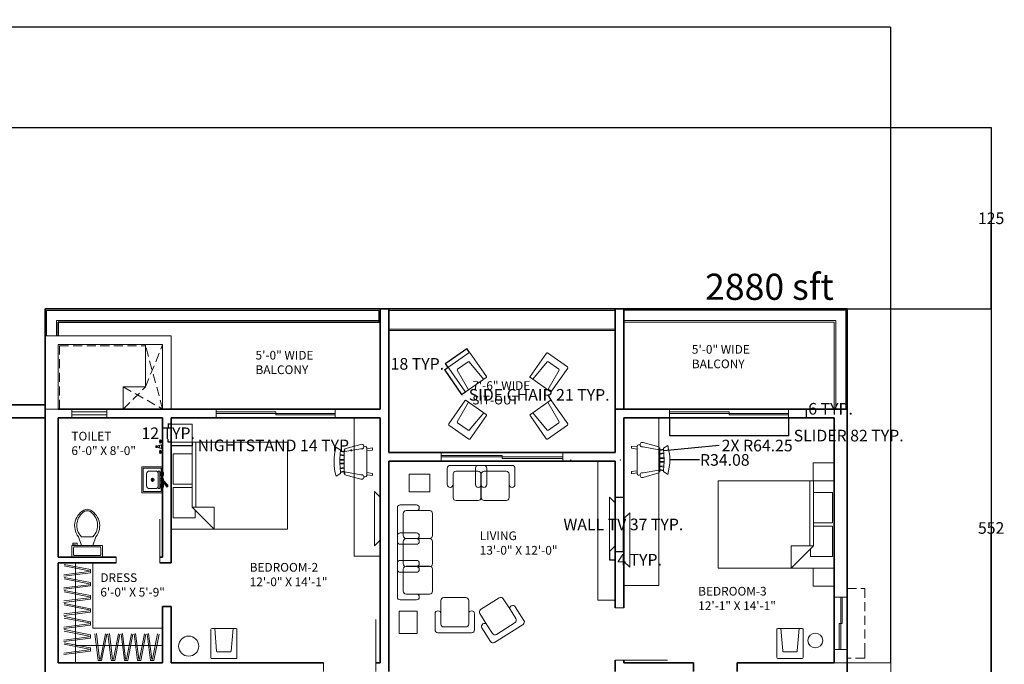
# Model space of a CAD drawing. Units: inches. Extents: x 3343 to 4790, y 1140 to 2641.
# Tile 10 of 10: x 4104 to 4782, y 2196 to 2641. Entities that reach past the tile are written whole.
import ezdxf

# ---------------------------------------------------------------- set-up
doc = ezdxf.new("R2010")
doc.units = ezdxf.units.IN
doc.header["$LTSCALE"] = 5
doc.header["$MEASUREMENT"] = 0
doc.linetypes.add('HIDDEN', pattern=[0.375, 0.25, -0.125])
for name, color, linetype, lineweight in [('A-ANNO-DIMS', 2, 'Continuous', 18), ('A-AREA-IDEN', 7, 'Continuous', 18), ('A-AREA-TAGS', 1, 'Continuous', 25), ('A-DOOR', 3, 'Continuous', 18), ('A-EQPM', 9, 'Continuous', 18), ('A-FLOR-CASE', 9, 'Continuous', 18), ('A-FLOR-FIXT', 9, 'Continuous', 18), ('A-FLOR-HIDN', 8, 'HIDDEN', 13), ('A-FLOR-RAIL', 7, 'Continuous', 18), ('A-FLOR-SHFT', 8, 'Continuous', 18), ('A-FURN', 8, 'Continuous', 13), ('A-GLAZ', 4, 'Continuous', 18), ('A-WALL', 7, 'Continuous', 35)]:
    doc.layers.add(name, color=color, linetype=linetype, lineweight=lineweight)
doc.styles.get("Standard").update_dxf_attribs({"font": 'arial.ttf'})
doc.dimstyles.get("Standard").update_dxf_attribs({"dimtxt": 8, "dimasz": 0.18, "dimexe": 0.18, "dimexo": 0.0625, "dimgap": 0.09, "dimtad": 0, "dimtih": 1, "dimtoh": 1, "dimdec": 1, "dimzin": 0, "dimdsep": 46, "dimlunit": 3, "dimtxsty": 'Standard', "dimcen": 0.09, "dimadec": 0, "dimazin": 0, "dimtfac": 1, "dimtdec": 1, "dimtofl": 0, "dimtmove": 0, "dimatfit": 3, "dimfxl": 1, "dimtolj": 1, "dimtzin": 0, "dimarcsym": 0})

# ---------------------------------------------------------------- blocks, each defined once
blk = doc.blocks.new('Toilet - top')
for p, q in [((9.5, -6), (9.5, -2)), ((-10, -8.5), (-8, -8.5)), ((-10, -9.5), (-10, -8.5)), ((-7, -9.5), (-10, -9.5)), ((-8, -8.5), (-8, -8)), ((-7, -8), (-7, -9.5)), ((-4, -8), (-6, -14)), ((4, -8), (6, -14)), ((4, -14), (-4, -14))]:
    blk.add_line(p, q)
blk.add_lwpolyline([(10.5, -8), (10.5, 0), (-10.5, 0), (-10.5, -8)], close=True)
for points in [[(-9.5, -2), (-9.5, -6)], [(8.5, -1), (-8.5, -1)], [(-8.5, -7), (8.5, -7)]]:
    blk.add_lwpolyline(points)
for centre, radius, start, end in [((-8.62, -1.88), 0.884, 81.8699, 188.1301), ((-8.62, -6.12), 0.884, 171.8699, 278.1301), ((8.62, -1.88), 0.884, 351.8699, 98.1301), ((8.62, -6.12), 0.884, 261.8699, 8.1301), ((3.52, -21.58), 12.17, 141.46911, 247.97143), ((4.2, -21.82), 11.33, 136.36773, 238.94682), ((-3.52, -21.58), 12.17, 292.02843, 38.53071), ((-4.2, -21.82), 11.33, 301.05301, 43.63209), ((0, -27.88), 4, 245.73182, 294.26817), ((0, -29), 4, 254.86053, 285.13947)]:
    blk.add_arc(centre, radius, start, end)
blk = doc.blocks.new('Faucet - Bathroom front')
for p, q in [((-5, 0), (-2.25, 0)), ((-4.5087, 0.25), (-2.7408, 0.25)), ((-4, 1.625), (-4.25, 1.625)), ((-4, 1.375), (-4.25, 1.375)), ((-3.1442, 0.75), (-4.0979, 0.75)), ((-3.25, 1.625), (-3, 1.625)), ((-3.25, 1.375), (-3, 1.375)), ((-1.5, 0), (1.5, 0)), ((-1, 0.5), (1, 0.5)), ((-0.5, 4.25), (0.5, 4.25)), ((0.5, 3.75), (-0.5, 3.75)), ((-0.5, 3), (0.5, 3)), ((0.5, 2), (-0.5, 2)), ((-0.25, 3), (-0.25, 3.5)), ((0.25, 3.5), (0.25, 3)), ((2.25, 0), (5, 0)), ((2.7413, 0.25), (4.5092, 0.25)), ((3.25, 1.625), (3, 1.625)), ((3.25, 1.375), (3, 1.375)), ((4.1058, 0.75), (3.1521, 0.75)), ((4, 1.625), (4.25, 1.625)), ((4, 1.375), (4.25, 1.375))]:
    blk.add_line(p, q)
for points in [[(-4, 1), (-4, 2), (-3.25, 2), (-3.25, 1)], [(3.25, 1), (3.25, 2), (4, 2), (4, 1)]]:
    blk.add_lwpolyline(points, close=True)
for points in [[(-0.5, 3.75), (-0.5, 4.25)], [(-0.25, 4.5), (0.25, 4.5)], [(0.25, 3.5), (-0.25, 3.5)], [(0.5, 4.25), (0.5, 3.75)]]:
    blk.add_lwpolyline(points)
for centre in [(-4.5, 1.5), (-3.625, 1.5), (-2.75, 1.5), (2.75, 1.5), (3.625, 1.5), (4.5, 1.5)]:
    blk.add_circle(centre, 0.2795)
for centre, radius, start, end in [((-5.375, 1.375), 1.4252, 285.2551, 344.7449), ((-1.875, 1.375), 1.4252, 195.2551, 254.7449), ((-0.7962, -0.2038), 0.7327, 106.1502, 163.8498), ((3, 1), 4.0311, 150.2551, 187.125), ((0.6413, 2.5), 1.246, 156.3417, 203.6583), ((-0.2575, 4.2575), 0.2426, 88.22243, 181.7776), ((-0.2575, 3.7425), 0.2426, 178.2224, 271.7776), ((0.2575, 4.2575), 0.2426, 358.2224, 91.77757), ((0.2575, 3.7425), 0.2426, 268.2224, 1.777565), ((-3, 1), 4.0311, 352.875, 29.74488), ((-0.6413, 2.5), 1.246, 336.3417, 23.65835), ((0.7962, -0.2038), 0.7327, 16.1502, 73.84979), ((1.875, 1.375), 1.4252, 285.2551, 344.7449), ((5.375, 1.375), 1.4252, 195.2551, 254.7449)]:
    blk.add_arc(centre, radius, start, end)
blk = doc.blocks.new('Faucet - kit sink front')
for p, q in [((-4.5, 1), (-4.5, 1.5)), ((-3.5, 1.5), (-3.5, 1)), ((-0.75, 3.5), (0.3192, 3.5)), ((-0.75, 1), (-0.75, 3.5)), ((-0.25, 3), (3.75, 6.5)), ((3.75, 6), (-0.25, 2.5)), ((-0.25, 2.5), (-0.25, 3)), ((0.75, 2.5), (-0.25, 2.5)), ((4.1921, 5.5041), (0.75, 2.5)), ((0.75, 2.5), (0.75, 1)), ((3.5, 1.5), (3.5, 1)), ((3.75, 6), (3.75, 6.5)), ((3.75, 6.5), (4.75, 6.5)), ((3.75, 5.5), (3.75, 6)), ((4.75, 6), (3.75, 6)), ((4.75, 5.5), (3.75, 5.5)), ((4.5, 1), (4.5, 1.5)), ((4.75, 6.5), (4.75, 6)), ((4.75, 6), (4.75, 5.5))]:
    blk.add_line(p, q)
for points in [[(-6, 0), (-6, 1), (6, 1), (6, 0)], [(-5.5, 2.5), (-5.5, 3.25), (-4.5, 3.25), (-4.5, 2.5)], [(5.5, 2.5), (5.5, 3.25), (4.5, 3.25), (4.5, 2.5)]]:
    blk.add_lwpolyline(points, close=True)
for points in [[(-5, 3.2513), (-5, 3.5), (-3, 3.5), (-3, 1.5), (-5, 1.5), (-5, 2.5)], [(5, 3.2513), (5, 3.5), (3, 3.5), (3, 1.5), (5, 1.5), (5, 2.5)]]:
    blk.add_lwpolyline(points)
blk = doc.blocks.new('Chair - Rocking')
for p, q in [((-8, -4.5), (-10, -1.5)), ((-7.5, -4.5), (-7, -7)), ((-6.5, -7), (-7.02225, -4.43)), ((-4.5, -7), (-4.96674, -4.19951)), ((-4, -7), (-4.40532, -4.16272)), ((-1.5, -4.05012), (-1.5, -7)), ((-1, -7), (-1, -4.05012)), ((1, -7), (1, -4.04655)), ((1.5, -4.05012), (1.5, -7)), ((4, -7), (4.40187, -4.18694)), ((4.5, -7), (4.96761, -4.19437)), ((6.5, -7), (7, -4.4057)), ((7.5, -4.5), (7, -7)), ((8, -4.5), (10, -1.5)), ((-9, -7.5), (-12, -18.49999)), ((-7, -7.5), (-9, -7.5)), ((-9, -18.49999), (-7, -7.5)), ((-8.23428, -6.99939), (-8.3093, -7.47958)), ((-8.23041, -7), (8.23915, -7)), ((7, -7.5), (9, -7.5)), ((9, -18.49999), (7, -7.5)), ((8.31071, -7.48854), (8.23449, -7.00073)), ((9, -7.5), (12, -18.49999)), ((-10.36644, -20.64523), (-10.5, -21.49999)), ((-9, -22.49999), (-9.5, -26.49999)), ((0, -22.49999), (-9.5, -22.49999)), ((-9.5, -26.49999), (-8, -26.49999)), ((-8, -26.49999), (-7.5, -22.49999)), ((0, -22.49999), (9.5, -22.49999)), ((8, -26.49999), (7.5, -22.49999)), ((9.5, -26.49999), (8, -26.49999)), ((9, -22.49999), (9.5, -26.49999)), ((10.5, -21.49999), (10.3575, -20.58798))]:
    blk.add_line(p, q)
for centre, radius, start, end in [((0, -34.08333), 34.08333, 72.93847, 107.0615), ((0, -68.25004), 64.25, 93.92211, 97.15267), ((0, -68.25004), 64.25, 82.84733, 93.92211), ((-10.5, -18.99999), 1.58114, 161.5651, 18.43495), ((10.5, -18.99999), 1.58114, 161.5651, 18.43495), ((-9.5, -21.49999), 1, 180, 270), ((9.5, -21.49999), 1, 270, 0)]:
    blk.add_arc(centre, radius, start, end)
blk = doc.blocks.new('Bed - Queen')
for p, q in [((0, -80.00003), (0, 0)), ((0, 0), (59.99999, 0)), ((59.99999, 0), (59.99999, -80.00003)), ((7.99999, -1.2), (28.79998, -1.2)), ((7.99999, -14.4), (7.99999, -1.2)), ((28.79998, -1.2), (28.79998, -14.4)), ((31.19999, -1.2), (51.99999, -1.2)), ((31.19999, -14.4), (31.19999, -1.2)), ((51.99999, -1.2), (51.99999, -16.4)), ((0, -14.4), (44.8, -14.4)), ((44.8, -16.8), (0, -16.8)), ((59.99999, -29.6), (44.8, -14.4)), ((44.8, -14.4), (44.8, -29.6)), ((51.99999, -16.4), (46.79936, -16.4)), ((44.8, -29.6), (59.99999, -29.6)), ((59.99999, -80.00003), (0, -80.00003))]:
    blk.add_line(p, q)
blk = doc.blocks.new('SOFA-3-SEAT')
for p, q in [((0, 63.51), (0, 40.3)), ((13.11, 65.51), (2, 65.51)), ((13.11, 61.51), (6, 61.51)), ((13.11, 61.51), (22.22, 61.51)), ((15.11, 63.51), (15.11, 63.51)), ((4, 59.51), (4, 44.3)), ((24.22, 44.3), (24.22, 59.51)), ((0, 44.2), (0, 20.98)), ((13.11, 46.2), (2, 46.2)), ((6, 42.3), (13.11, 42.3)), ((13.11, 42.2), (6, 42.2)), ((13.11, 42.3), (22.22, 42.3)), ((13.11, 42.2), (22.22, 42.2)), ((15.11, 44.2), (15.11, 44.2)), ((2, 38.3), (13.11, 38.3)), ((4, 40.2), (4, 24.98)), ((15.11, 40.3), (15.11, 40.3)), ((24.22, 24.98), (24.22, 40.2)), ((13.11, 27.21), (2, 27.21)), ((0, 25.21), (0, 2)), ((4, 21.21), (4, 6)), ((13.11, 23.21), (6, 23.21)), ((6, 22.98), (13.11, 22.98)), ((13.11, 23.21), (22.22, 23.21)), ((13.11, 22.98), (22.22, 22.98)), ((15.11, 25.21), (15.11, 25.21)), ((15.11, 20.98), (15.11, 20.98)), ((24.22, 6), (24.22, 21.21)), ((2, 18.98), (13.11, 18.98)), ((2, 0), (13.11, 0)), ((6, 4), (13.11, 4)), ((13.11, 4), (22.22, 4)), ((15.11, 2), (15.11, 2))]:
    blk.add_line(p, q)
for centre, start, end in [((2, 63.51), 90, 180), ((6, 59.51), 90, 180), ((13.11, 63.51), 0, 90), ((13.11, 63.51), 270, 0), ((22.22, 59.51), 0, 90), ((2, 44.2), 90, 180), ((6, 44.3), 180, 270), ((6, 40.2), 90, 180), ((13.11, 44.2), 0, 90), ((13.11, 44.2), 270, 0), ((13.11, 40.3), 0, 90), ((22.22, 44.3), 270, 0), ((22.22, 40.2), 0, 90), ((2, 40.3), 180, 270), ((13.11, 40.3), 270, 0), ((2, 25.21), 90, 180), ((13.11, 25.21), 0, 90), ((2, 20.98), 180, 270), ((6, 24.98), 180, 270), ((6, 21.21), 90, 180), ((13.11, 25.21), 270, 0), ((13.11, 20.98), 0, 90), ((13.11, 20.98), 270, 0), ((22.22, 24.98), 270, 0), ((22.22, 21.21), 0, 90), ((2, 2), 180, 270), ((6, 6), 180, 270), ((13.11, 2), 0, 90), ((13.11, 2), 270, 0), ((22.22, 6), 270, 0)]:
    blk.add_arc(centre, 2, start, end)
blk = doc.blocks.new('SOFA-2-SEAT')
for p, q in [((0, 22.22), (0, 11.11)), ((25.21, 24.22), (2, 24.22)), ((19.41, 22.22), (19.41, 11.11)), ((44.62, 24.22), (21.41, 24.22)), ((27.21, 11.11), (27.21, 22.22)), ((46.62, 11.11), (46.62, 22.22)), ((4, 18.22), (4, 11.11)), ((21.21, 20.22), (6, 20.22)), ((23.21, 11.11), (23.21, 18.22)), ((23.41, 18.22), (23.41, 11.11)), ((40.62, 20.22), (25.41, 20.22)), ((42.62, 11.11), (42.62, 18.22)), ((2, 9.11), (2, 9.11)), ((4, 11.11), (4, 2)), ((21.41, 9.11), (21.41, 9.11)), ((23.21, 11.11), (23.21, 2)), ((23.41, 11.11), (23.41, 2)), ((25.21, 9.11), (25.21, 9.11)), ((42.62, 11.11), (42.62, 2)), ((44.62, 9.11), (44.62, 9.11)), ((6, 0), (21.21, 0)), ((25.41, 0), (40.62, 0))]:
    blk.add_line(p, q)
for centre, start, end in [((2, 22.22), 90, 180), ((21.41, 22.22), 90, 180), ((25.21, 22.22), 0, 90), ((44.62, 22.22), 0, 90), ((6, 18.22), 90, 180), ((21.21, 18.22), 0, 90), ((25.41, 18.22), 90, 180), ((40.62, 18.22), 0, 90), ((2, 11.11), 180, 270), ((2, 11.11), 270, 0), ((21.41, 11.11), 180, 270), ((21.41, 11.11), 270, 0), ((25.21, 11.11), 180, 270), ((25.21, 11.11), 270, 0), ((44.62, 11.11), 180, 270), ((44.62, 11.11), 270, 0), ((6, 2), 180, 270), ((21.21, 2), 270, 0), ((25.41, 2), 180, 270), ((40.62, 2), 270, 0)]:
    blk.add_arc(centre, 2, start, end)
blk = doc.blocks.new('LOUNGE-CHAIR')
for p, q in [((4, 13.11), (4, 22.22)), ((6, 24.22), (21.21, 24.22)), ((23.21, 13.11), (23.21, 22.22)), ((2, 15.11), (2, 15.11)), ((25.21, 15.11), (25.21, 15.11)), ((0, 2), (0, 13.11)), ((4, 6), (4, 13.11)), ((23.21, 13.11), (23.21, 6)), ((27.21, 13.11), (27.21, 2)), ((21.21, 4), (6, 4)), ((25.21, 0), (2, 0))]:
    blk.add_line(p, q)
for centre, start, end in [((6, 22.22), 90, 180), ((21.21, 22.22), 0, 90), ((2, 13.11), 90, 180), ((2, 13.11), 0, 90), ((25.21, 13.11), 90, 180), ((25.21, 13.11), 0, 90), ((2, 2), 180, 270), ((6, 6), 180, 270), ((21.21, 6), 270, 0), ((25.21, 2), 270, 0)]:
    blk.add_arc(centre, 2, start, end)
blk = doc.blocks.new('CHAIR-SIDE')
for p, q in [((0.6, 20.7), (17.39, 20.7)), ((2.68, 20.7), (3.95, 5.17)), ((15.31, 20.7), (14.03, 5.17)), ((0, 0.6), (0, 20.1)), ((17.98, 20.1), (17.98, 0.6)), ((17.39, 0), (0.6, 0)), ((13.44, 4.62), (4.54, 4.62))]:
    blk.add_line(p, q)
for centre, start, end in [((0.6, 20.1), 90, 180), ((17.39, 20.1), 0, 90), ((0.6, 0.6), 180, 270), ((4.54, 5.22), 184.67931, 270), ((13.44, 5.22), 270, 355.32069), ((17.39, 0.6), 270, 0)]:
    blk.add_arc(centre, 0.595, start, end)
blk = doc.blocks.new('TV-WALL-MOUNT')
for p, q in [((0, 37.4), (4.02, 33.55)), ((0, 0), (4.02, 3.86))]:
    blk.add_line(p, q)
for points in [[(0, 37.4), (0, 0)], [(4.02, 0), (4.02, 37.4)]]:
    blk.add_lwpolyline(points)
blk = doc.blocks.new('WINDOW-82IN-SLIDING')
for p, q in [((0, 0), (0, 6)), ((0, 4), (41, 4)), ((0, 3), (82, 3)), ((41, 2), (41, 4)), ((41, 2), (82, 2)), ((82, 0), (82, 6))]:
    blk.add_line(p, q)
blk = doc.blocks.new('DOOR-36IN-6IN-JAMB')
for p, q in [((0, 30), (0, 36)), ((36, 30), (36, 36)), ((36, 36), (36, 0))]:
    blk.add_line(p, q)
blk = doc.blocks.new('DOOR-30IN-4IN-JAMB')
for p, q in [((30, 30), (0, 30)), ((26, 30), (30, 30)), ((26, 0), (30, 0))]:
    blk.add_line(p, q)
blk = doc.blocks.new('WARDROBE-HANGER')
for points in [[(0.22, 7.19), (17.51, 3.78), (17.51, 3.18), (0, 0.99)], [(0.41, 8.17), (18.51, 4.61), (18.51, 2.3), (0.12, 0)]]:
    blk.add_lwpolyline(points)
blk = doc.blocks.new('NIGHTSTAND')
blk.add_lwpolyline([(12.43, 0), (0, 0), (0, 14.43), (12.43, 14.43)], close=True)
blk = doc.blocks.new('*D31')
at = {"layer": 'A-ANNO-DIMS', "color": 0, "lineweight": -2, "ltscale": 5, "transparency": 16777216}
for p, q in [((4399, 2400.82), (4396.36, 2398.98)), ((4396.61, 2398.93), (4408.25, 2382.26)), ((4410.85, 2383.85), (4408.21, 2382.01)), ((4408.36, 2382.11), (4408.46, 2381.96)), ((4408.46, 2381.96), (4408.64, 2381.96))]:
    blk.add_line(p, q, dxfattribs=at)
at = {"layer": 'A-ANNO-DIMS', "color": 0, "ltscale": 5, "transparency": 16777216}
for points in [[(4396.63, 2398.95), (4396.59, 2398.92), (4396.51, 2399.08)], [(4408.28, 2382.28), (4408.23, 2382.24), (4408.36, 2382.11)]]:
    blk.add_solid(points, dxfattribs=at)
at = {"layer": 'Defpoints', "color": 0, "ltscale": 5, "transparency": 16777216}
for p in [(4399.05, 2400.86), (4410.9, 2383.89), (4408.36, 2382.11)]:
    blk.add_point(p, dxfattribs=at)
at = {"layer": 'A-ANNO-DIMS', "color": 0, "ltscale": 5, "transparency": 16777216, "insert": (4461.71, 2381.96), "char_height": 8, "attachment_point": 5}
blk.add_mtext('\\A1;SIDE CHAIR 21 TYP.', dxfattribs=at)
blk = doc.blocks.new('*D32')
at = {"layer": 'A-ANNO-DIMS', "color": 0, "lineweight": -2, "ltscale": 5, "transparency": 16777216}
for p, q in [((4411.87, 2413.6), (4397.42, 2403.51)), ((4413.76, 2411.21), (4411.92, 2413.85)), ((4397.13, 2403.3), (4396.95, 2403.3)), ((4397.27, 2403.4), (4397.13, 2403.3)), ((4399.02, 2400.91), (4397.17, 2403.55))]:
    blk.add_line(p, q, dxfattribs=at)
at = {"layer": 'A-ANNO-DIMS', "color": 0, "ltscale": 5, "transparency": 16777216}
for points in [[(4411.85, 2413.62), (4411.89, 2413.57), (4412.02, 2413.7)], [(4397.4, 2403.53), (4397.44, 2403.48), (4397.27, 2403.4)]]:
    blk.add_solid(points, dxfattribs=at)
at = {"layer": 'Defpoints', "color": 0, "ltscale": 5, "transparency": 16777216}
for p in [(4413.8, 2411.15), (4397.27, 2403.4), (4399.05, 2400.86)]:
    blk.add_point(p, dxfattribs=at)
at = {"layer": 'A-ANNO-DIMS', "color": 0, "ltscale": 5, "transparency": 16777216, "insert": (4377.76, 2403.3), "char_height": 8, "attachment_point": 5}
blk.add_mtext('\\A1;18 TYP.', dxfattribs=at)
blk = doc.blocks.new('*D37')
at = {"layer": 'A-ANNO-DIMS', "color": 0, "lineweight": -2, "ltscale": 5, "transparency": 16777216}
for p, q in [((4208.13, 2349.2), (4208.13, 2346.92)), ((4222.56, 2349.2), (4222.56, 2346.92)), ((4208.31, 2347.1), (4222.38, 2347.1)), ((4222.56, 2347.1), (4222.74, 2347.1))]:
    blk.add_line(p, q, dxfattribs=at)
at = {"layer": 'A-ANNO-DIMS', "color": 0, "ltscale": 5, "transparency": 16777216}
for points in [[(4208.31, 2347.13), (4208.31, 2347.07), (4208.13, 2347.1)], [(4222.38, 2347.13), (4222.38, 2347.07), (4222.56, 2347.1)]]:
    blk.add_solid(points, dxfattribs=at)
at = {"layer": 'Defpoints', "color": 0, "ltscale": 5, "transparency": 16777216}
for p in [(4208.13, 2349.27), (4222.56, 2349.27), (4222.56, 2347.1)]:
    blk.add_point(p, dxfattribs=at)
at = {"layer": 'A-ANNO-DIMS', "color": 0, "ltscale": 5, "transparency": 16777216, "insert": (4279.98, 2347.1), "char_height": 8, "attachment_point": 5}
blk.add_mtext('\\A1;NIGHTSTAND 14 TYP.', dxfattribs=at)
blk = doc.blocks.new('*D38')
at = {"layer": 'A-ANNO-DIMS', "color": 0, "lineweight": -2, "ltscale": 5, "transparency": 16777216}
for p, q in [((4208.07, 2361.69), (4205.78, 2361.69)), ((4205.96, 2361.51), (4205.96, 2359.59)), ((4208.07, 2349.27), (4205.78, 2349.27)), ((4205.96, 2349.45), (4205.96, 2351.37))]:
    blk.add_line(p, q, dxfattribs=at)
at = {"layer": 'A-ANNO-DIMS', "color": 0, "ltscale": 5, "transparency": 16777216}
for points in [[(4205.93, 2361.51), (4205.99, 2361.51), (4205.96, 2361.69)], [(4205.93, 2349.45), (4205.99, 2349.45), (4205.96, 2349.27)]]:
    blk.add_solid(points, dxfattribs=at)
at = {"layer": 'Defpoints', "color": 0, "ltscale": 5, "transparency": 16777216}
for p in [(4208.13, 2361.69), (4205.96, 2349.27), (4208.13, 2349.27)]:
    blk.add_point(p, dxfattribs=at)
at = {"layer": 'A-ANNO-DIMS', "color": 0, "ltscale": 5, "transparency": 16777216, "insert": (4205.96, 2355.48), "char_height": 8, "attachment_point": 5}
blk.add_mtext('\\A1;12 TYP.', dxfattribs=at)
blk = doc.blocks.new('*D45')
at = {"layer": 'A-ANNO-DIMS', "color": 0, "lineweight": -2, "ltscale": 5, "transparency": 16777216}
for p, q in [((4514.19, 2311.31), (4519.92, 2311.31)), ((4519.74, 2311.13), (4519.74, 2296.79)), ((4519.74, 2274.09), (4519.74, 2288.43)), ((4514.19, 2273.91), (4519.92, 2273.91))]:
    blk.add_line(p, q, dxfattribs=at)
at = {"layer": 'A-ANNO-DIMS', "color": 0, "ltscale": 5, "transparency": 16777216}
for points in [[(4519.71, 2311.13), (4519.77, 2311.13), (4519.74, 2311.31)], [(4519.71, 2274.09), (4519.77, 2274.09), (4519.74, 2273.91)]]:
    blk.add_solid(points, dxfattribs=at)
at = {"layer": 'Defpoints', "color": 0, "ltscale": 5, "transparency": 16777216}
for p in [(4514.13, 2311.31), (4519.74, 2311.31), (4514.13, 2273.91)]:
    blk.add_point(p, dxfattribs=at)
at = {"layer": 'A-ANNO-DIMS', "color": 0, "ltscale": 5, "transparency": 16777216, "insert": (4519.74, 2292.61), "char_height": 8, "attachment_point": 5}
blk.add_mtext('\\A1;WALL TV 37 TYP.', dxfattribs=at)
blk = doc.blocks.new('*D46')
at = {"layer": 'A-ANNO-DIMS', "color": 0, "lineweight": -2, "ltscale": 5, "transparency": 16777216}
for p, q in [((4510.11, 2273.84), (4510.11, 2268.12)), ((4510.29, 2268.3), (4513.95, 2268.3)), ((4514.13, 2273.84), (4514.13, 2268.12)), ((4514.13, 2268.3), (4514.31, 2268.3))]:
    blk.add_line(p, q, dxfattribs=at)
at = {"layer": 'A-ANNO-DIMS', "color": 0, "ltscale": 5, "transparency": 16777216}
for points in [[(4510.29, 2268.33), (4510.29, 2268.27), (4510.11, 2268.3)], [(4513.95, 2268.33), (4513.95, 2268.27), (4514.13, 2268.3)]]:
    blk.add_solid(points, dxfattribs=at)
at = {"layer": 'Defpoints', "color": 0, "ltscale": 5, "transparency": 16777216}
for p in [(4510.11, 2273.91), (4514.13, 2273.91), (4514.13, 2268.3)]:
    blk.add_point(p, dxfattribs=at)
at = {"layer": 'A-ANNO-DIMS', "color": 0, "ltscale": 5, "transparency": 16777216, "insert": (4530.92, 2268.3), "char_height": 8, "attachment_point": 5}
blk.add_mtext('\\A1;4 TYP.', dxfattribs=at)
blk = doc.blocks.new('*D75')
at = {"layer": 'A-ANNO-DIMS', "color": 0, "lineweight": -2, "ltscale": 5, "transparency": 16777216}
for p, q in [((4551.63, 2366.1), (4551.63, 2353.68)), ((4633.63, 2366.1), (4633.63, 2353.68)), ((4551.81, 2353.86), (4633.45, 2353.86)), ((4633.63, 2353.86), (4633.81, 2353.86))]:
    blk.add_line(p, q, dxfattribs=at)
at = {"layer": 'A-ANNO-DIMS', "color": 0, "ltscale": 5, "transparency": 16777216}
for points in [[(4551.81, 2353.89), (4551.81, 2353.83), (4551.63, 2353.86)], [(4633.45, 2353.89), (4633.45, 2353.83), (4633.63, 2353.86)]]:
    blk.add_solid(points, dxfattribs=at)
at = {"layer": 'Defpoints', "color": 0, "ltscale": 5, "transparency": 16777216}
for p in [(4551.63, 2366.16), (4633.63, 2366.16), (4633.63, 2353.86)]:
    blk.add_point(p, dxfattribs=at)
at = {"layer": 'A-ANNO-DIMS', "color": 0, "ltscale": 5, "transparency": 16777216, "insert": (4675.09, 2353.86), "char_height": 8, "attachment_point": 5}
blk.add_mtext('\\A1;SLIDER 82 TYP.', dxfattribs=at)
blk = doc.blocks.new('*D76')
at = {"layer": 'A-ANNO-DIMS', "color": 0, "lineweight": -2, "ltscale": 5, "transparency": 16777216}
for p, q in [((4633.69, 2372.16), (4646.11, 2372.16)), ((4645.93, 2372.16), (4645.93, 2372.34)), ((4645.93, 2372.34), (4646.11, 2372.34)), ((4645.93, 2366.34), (4645.93, 2371.98)), ((4633.69, 2366.16), (4646.11, 2366.16))]:
    blk.add_line(p, q, dxfattribs=at)
at = {"layer": 'A-ANNO-DIMS', "color": 0, "ltscale": 5, "transparency": 16777216}
for points in [[(4645.9, 2371.98), (4645.96, 2371.98), (4645.93, 2372.16)], [(4645.9, 2366.34), (4645.96, 2366.34), (4645.93, 2366.16)]]:
    blk.add_solid(points, dxfattribs=at)
at = {"layer": 'Defpoints', "color": 0, "ltscale": 5, "transparency": 16777216}
for p in [(4633.63, 2372.16), (4645.93, 2372.16), (4633.63, 2366.16)]:
    blk.add_point(p, dxfattribs=at)
at = {"layer": 'A-ANNO-DIMS', "color": 0, "ltscale": 5, "transparency": 16777216, "insert": (4662.58, 2372.34), "char_height": 8, "attachment_point": 5}
blk.add_mtext('\\A1;6 TYP.', dxfattribs=at)
blk = doc.blocks.new('*D83')
at = {"layer": 'A-ANNO-DIMS', "color": 0, "lineweight": -2, "ltscale": 5, "transparency": 16777216}
for p, q in [((3424.13, 2432.05), (3424.13, 2635.49)), ((3424.31, 2635.31), (4052.48, 2635.31)), ((4703.95, 2635.31), (4075.77, 2635.31)), ((4704.13, 2197.22), (4704.13, 2635.49))]:
    blk.add_line(p, q, dxfattribs=at)
at = {"layer": 'A-ANNO-DIMS', "color": 0, "ltscale": 5, "transparency": 16777216}
for points in [[(3424.31, 2635.34), (3424.31, 2635.28), (3424.13, 2635.31)], [(4703.95, 2635.34), (4703.95, 2635.28), (4704.13, 2635.31)]]:
    blk.add_solid(points, dxfattribs=at)
at = {"layer": 'Defpoints', "color": 0, "ltscale": 5, "transparency": 16777216}
for p in [(4704.13, 2635.31), (3424.13, 2431.99), (4704.13, 2197.16)]:
    blk.add_point(p, dxfattribs=at)
at = {"layer": 'A-ANNO-DIMS', "color": 0, "ltscale": 5, "transparency": 16777216, "insert": (4064.13, 2635.31), "char_height": 8, "attachment_point": 5}
blk.add_mtext('\\A1;1280', dxfattribs=at)
blk = doc.blocks.new('*D87')
at = {"layer": 'A-ANNO-DIMS', "color": 0, "lineweight": -2, "ltscale": 5, "transparency": 16777216}
for p, q in [((3977.19, 2566.16), (4773.46, 2566.16)), ((4773.28, 2565.98), (4773.28, 2294.34)), ((4773.28, 2014.34), (4773.28, 2285.99)), ((3977.19, 2014.16), (4773.46, 2014.16))]:
    blk.add_line(p, q, dxfattribs=at)
at = {"layer": 'A-ANNO-DIMS', "color": 0, "ltscale": 5, "transparency": 16777216}
for points in [[(4773.25, 2565.98), (4773.31, 2565.98), (4773.28, 2566.16)], [(4773.25, 2014.34), (4773.31, 2014.34), (4773.28, 2014.16)]]:
    blk.add_solid(points, dxfattribs=at)
at = {"layer": 'Defpoints', "color": 0, "ltscale": 5, "transparency": 16777216}
for p in [(3977.13, 2566.16), (3977.13, 2014.16), (4773.28, 2014.16)]:
    blk.add_point(p, dxfattribs=at)
at = {"layer": 'A-ANNO-DIMS', "color": 0, "ltscale": 5, "transparency": 16777216, "insert": (4773.28, 2290.16), "char_height": 8, "attachment_point": 5}
blk.add_mtext('\\A1;552', dxfattribs=at)
blk = doc.blocks.new('*D88')
at = {"layer": 'A-ANNO-DIMS', "color": 0, "lineweight": -2, "ltscale": 5, "transparency": 16777216}
for p, q in [((4674.19, 2441.16), (4773.46, 2441.16)), ((4773.28, 2440.98), (4773.28, 2150.34)), ((4773.28, 1851.34), (4773.28, 2141.99)), ((4674.19, 1851.16), (4773.46, 1851.16))]:
    blk.add_line(p, q, dxfattribs=at)
at = {"layer": 'A-ANNO-DIMS', "color": 0, "ltscale": 5, "transparency": 16777216}
for points in [[(4773.25, 2440.98), (4773.31, 2440.98), (4773.28, 2441.16)], [(4773.25, 1851.34), (4773.31, 1851.34), (4773.28, 1851.16)]]:
    blk.add_solid(points, dxfattribs=at)
at = {"layer": 'Defpoints', "color": 0, "ltscale": 5, "transparency": 16777216}
for p in [(4674.13, 2441.16), (4773.28, 2441.16), (4674.13, 1851.16)]:
    blk.add_point(p, dxfattribs=at)
at = {"layer": 'A-ANNO-DIMS', "color": 0, "ltscale": 5, "transparency": 16777216, "insert": (4773.28, 2146.16), "char_height": 8, "attachment_point": 5}
blk.add_mtext('\\A1;590', dxfattribs=at)
blk = doc.blocks.new('*D89')
at = {"layer": 'A-ANNO-DIMS', "color": 0, "lineweight": -2, "ltscale": 5, "transparency": 16777216}
for p, q in [((3977.19, 2566.16), (4773.46, 2566.16)), ((4773.28, 2565.98), (4773.28, 2507.84)), ((4773.28, 2441.34), (4773.28, 2499.49)), ((4121.19, 2441.16), (4773.46, 2441.16))]:
    blk.add_line(p, q, dxfattribs=at)
at = {"layer": 'A-ANNO-DIMS', "color": 0, "ltscale": 5, "transparency": 16777216}
for points in [[(4773.25, 2565.98), (4773.31, 2565.98), (4773.28, 2566.16)], [(4773.25, 2441.34), (4773.31, 2441.34), (4773.28, 2441.16)]]:
    blk.add_solid(points, dxfattribs=at)
at = {"layer": 'Defpoints', "color": 0, "ltscale": 5, "transparency": 16777216}
for p in [(3977.13, 2566.16), (4121.13, 2441.16), (4773.28, 2441.16)]:
    blk.add_point(p, dxfattribs=at)
at = {"layer": 'A-ANNO-DIMS', "color": 0, "ltscale": 5, "transparency": 16777216, "insert": (4773.28, 2503.66), "char_height": 8, "attachment_point": 5}
blk.add_mtext('\\A1;125', dxfattribs=at)
blk = doc.blocks.new('*D99')
at = {"layer": 'A-ANNO-DIMS', "color": 0, "lineweight": -2, "ltscale": 5, "transparency": 16777216}
for p, q in [((4585.89, 2347), (4547.7, 2343.3)), ((4483.48, 2337.08), (4483.66, 2337.08)), ((4483.57, 2336.99), (4483.57, 2337.17))]:
    blk.add_line(p, q, dxfattribs=at)
at = {"layer": 'A-ANNO-DIMS', "color": 0, "ltscale": 5, "transparency": 16777216}
blk.add_solid([(4547.69, 2343.33), (4547.7, 2343.27), (4547.52, 2343.28)], dxfattribs=at)
at = {"layer": 'Defpoints', "color": 0, "ltscale": 5, "transparency": 16777216}
for p in [(4547.52, 2343.28), (4483.57, 2337.08)]:
    blk.add_point(p, dxfattribs=at)
at = {"layer": 'A-ANNO-DIMS', "color": 0, "ltscale": 5, "transparency": 16777216, "insert": (4612, 2347), "char_height": 8, "attachment_point": 5}
blk.add_mtext('\\A1;2X R64.25', dxfattribs=at)
blk = doc.blocks.new('*D100')
at = {"layer": 'A-ANNO-DIMS', "color": 0, "lineweight": -2, "ltscale": 5, "transparency": 16777216}
for p, q in [((4517.64, 2337.08), (4517.82, 2337.08)), ((4517.73, 2336.99), (4517.73, 2337.17)), ((4572.27, 2337.09), (4552, 2337.09))]:
    blk.add_line(p, q, dxfattribs=at)
at = {"layer": 'A-ANNO-DIMS', "color": 0, "ltscale": 5, "transparency": 16777216}
blk.add_solid([(4552, 2337.12), (4552, 2337.06), (4551.82, 2337.09)], dxfattribs=at)
at = {"layer": 'Defpoints', "color": 0, "ltscale": 5, "transparency": 16777216}
for p in [(4517.73, 2337.08), (4551.82, 2337.09)]:
    blk.add_point(p, dxfattribs=at)
at = {"layer": 'A-ANNO-DIMS', "color": 0, "ltscale": 5, "transparency": 16777216, "insert": (4589.69, 2337.09), "char_height": 8, "attachment_point": 5}
blk.add_mtext('\\A1;R34.08', dxfattribs=at)

msp = doc.modelspace()

# ---------------------------------------------------------------- linework, layer by layer
at = {"layer": 'A-FLOR-CASE'}
for p, q in [((4334.13, 2366.161), (4334.13, 2270.79)), ((4544.13, 2366.161), (4544.13, 2250.504)), ((4502.13, 2336.161), (4502.13, 2240.349)), ((4334.13, 2270.79), (4352.13, 2270.79)), ((4142.13, 2266.161), (4142.13, 2197.161)), ((4142.13, 2266.161), (4142.13, 2197.161)), ((4154.13, 2266.161), (4154.13, 2221.161)), ((4520.13, 2250.504), (4544.13, 2250.504)), ((4514.13, 2240.349), (4502.13, 2240.349)), ((4154.13, 2221.161), (4202.13, 2221.161)), ((4142.13, 2209.161), (4202.13, 2209.161))]:
    msp.add_line(p, q, dxfattribs=at)
at = {"layer": 'A-FLOR-FIXT'}
for p, q in [((4196.277, 2323.371), (4194.158, 2323.371)), ((4195.218, 2324.431), (4195.218, 2322.312))]:
    msp.add_line(p, q, dxfattribs=at)
for points in [[(4202.13, 2314.34), (4187.693, 2314.34), (4187.693, 2332.403), (4202.13, 2332.403)], [(4188.693, 2315.34), (4188.693, 2331.403), (4201.13, 2331.403), (4201.13, 2315.34)]]:
    msp.add_lwpolyline(points, close=True, dxfattribs=at)
msp.add_lwpolyline([(4197.13, 2329.403), (4193.13, 2329.403, 0.4142136), (4191.13, 2327.403), (4191.13, 2319.34, 0.4142136), (4193.13, 2317.34), (4197.13, 2317.34, 0.4142136), (4199.13, 2319.34), (4199.13, 2327.403, 0.4142136)], format="xyb", close=True, dxfattribs=at)
msp.add_circle((4195.218, 2323.371), 1.06, dxfattribs=at)
at = {"layer": 'A-FLOR-HIDN', "ltscale": 5}
for p, q in [((4190.366, 2387.422), (4202.13, 2416.603)), ((4131.042, 2372.161), (4131.042, 2415.682)), ((4131.042, 2415.682), (4190.366, 2415.682)), ((4202.13, 2372.161), (4190.366, 2415.682)), ((4175.047, 2387.422), (4202.13, 2372.161)), ((4175.047, 2372.161), (4190.366, 2387.422)), ((4674.13, 2242.38), (4674.13, 2248.38)), ((4674.13, 2248.38), (4686.13, 2248.38)), ((4686.13, 2248.38), (4686.13, 2206.38)), ((4686.13, 2206.38), (4686.13, 2200.38)), ((4686.13, 2200.38), (4674.13, 2200.38))]:
    msp.add_line(p, q, dxfattribs=at)
at = {"layer": 'A-FLOR-RAIL'}
for p, q in [((4358.13, 2441.161), (4358.13, 2440.161)), ((4358.13, 2440.161), (4514.13, 2440.161)), ((4129.053, 2422.603), (4129.053, 2433.238)), ((4129.053, 2433.238), (4344.206, 2433.238)), ((4344.206, 2433.238), (4351.13, 2433.238)), ((4352.13, 2432.161), (4351.13, 2432.161)), ((4358.13, 2427.333), (4514.13, 2427.333)), ((4358.13, 2426.333), (4514.13, 2426.333)), ((4121.13, 2422.603), (4122.13, 2422.603))]:
    msp.add_line(p, q, dxfattribs=at)
for points in [[(4122.13, 2422.603), (4122.13, 2440.161), (4351.13, 2440.161), (4351.13, 2432.161)], [(4520.13, 2440.261), (4673.23, 2440.261), (4673.23, 2372.161)], [(4520.13, 2433.161), (4666.13, 2433.161), (4666.13, 2372.161)], [(4520.13, 2432.161), (4665.13, 2432.161), (4665.13, 2372.161)]]:
    msp.add_lwpolyline(points, dxfattribs=at)
at = {"layer": 'A-FLOR-SHFT'}
for p, q in [((4130.13, 2416.603), (4130.13, 2372.161)), ((4190.366, 2416.603), (4190.366, 2387.422)), ((4190.366, 2387.422), (4175.047, 2387.422)), ((4175.047, 2387.422), (4175.047, 2372.161)), ((4130.13, 2372.161), (4121.13, 2372.161)), ((4208.13, 2372.161), (4208.13, 2374.174)), ((4665.13, 2197.161), (4674.13, 2197.161)), ((4674.13, 2197.161), (4704.13, 2197.161)), ((4704.13, 2197.161), (4704.13, 2077.161))]:
    msp.add_line(p, q, dxfattribs=at)
for points in [[(4208.13, 2372.161), (4208.13, 2422.603), (4121.13, 2422.603)], [(4202.13, 2372.161), (4202.13, 2416.603), (4130.13, 2416.603)]]:
    msp.add_lwpolyline(points, dxfattribs=at)
at = {"layer": 'A-FURN'}
for points in [[(4372.139, 2327.358), (4386.248, 2327.358), (4386.248, 2315.165), (4372.139, 2315.165)], [(4365.105, 2232.868), (4377.718, 2232.868), (4377.718, 2217.543), (4365.105, 2217.543)]]:
    msp.add_lwpolyline(points, close=True, dxfattribs=at)
for centre, radius in [((4220.1, 2208.744), 6.927), ((4652.065, 2212.632), 5.088)]:
    msp.add_circle(centre, radius, dxfattribs=at)
at = {"layer": 'A-GLAZ'}
for p, q in [((4139.596, 2372.161), (4139.596, 2366.161)), ((4139.596, 2370.161), (4163.596, 2370.161)), ((4163.596, 2372.161), (4163.596, 2366.161)), ((4139.596, 2368.161), (4163.596, 2368.161)), ((4394.13, 2336.161), (4394.13, 2342.161)), ((4478.13, 2336.161), (4478.13, 2342.161)), ((4394.13, 2340.161), (4436.13, 2340.161)), ((4394.13, 2339.161), (4478.13, 2339.161)), ((4436.13, 2338.161), (4436.13, 2340.161)), ((4436.13, 2338.161), (4478.13, 2338.161)), ((4665.13, 2242.38), (4674.13, 2242.38)), ((4669.63, 2242.38), (4669.63, 2206.38)), ((4670.63, 2242.38), (4670.63, 2224.38)), ((4668.63, 2224.38), (4670.63, 2224.38)), ((4668.63, 2224.38), (4668.63, 2206.38)), ((4665.13, 2206.38), (4674.13, 2206.38))]:
    msp.add_line(p, q, dxfattribs=at)
at = {"layer": 'A-WALL'}
for p, q in [((4121.13, 2441.161), (4121.13, 2167.871)), ((4121.13, 2441.161), (4674.13, 2441.161)), ((4352.13, 2441.161), (4352.13, 2372.161)), ((4358.13, 2441.161), (4358.13, 2342.161)), ((4514.13, 2441.161), (4514.13, 2342.161)), ((4520.13, 2441.161), (4520.13, 2372.161)), ((4674.13, 2441.161), (4674.13, 1851.161)), ((4130.13, 2432.161), (4130.13, 2422.603)), ((4130.13, 2432.161), (4352.13, 2432.161)), ((4121.13, 2375.161), (3977.13, 2375.161)), ((4130.13, 2372.161), (4352.13, 2372.161)), ((4514.13, 2372.161), (4674.13, 2372.161)), ((4121.13, 2366.161), (3977.13, 2366.161)), ((4130.13, 2366.161), (4202.13, 2366.161)), ((4130.13, 2366.161), (4130.13, 2270.161)), ((4202.13, 2366.161), (4202.13, 2270.161)), ((4208.13, 2366.161), (4208.13, 2266.161)), ((4208.13, 2366.161), (4352.13, 2366.161)), ((4352.13, 2366.161), (4352.13, 2197.161)), ((4520.13, 2366.161), (4665.13, 2366.161)), ((4520.13, 2366.161), (4520.13, 2235.161)), ((4665.13, 2366.161), (4665.13, 2197.161)), ((4358.13, 2342.161), (4514.13, 2342.161)), ((4358.13, 2336.161), (4514.13, 2336.161)), ((4358.13, 2336.161), (4358.13, 2191.161)), ((4514.13, 2336.161), (4514.13, 2235.161)), ((4130.13, 2270.161), (4170.13, 2270.161)), ((4200.13, 2270.161), (4202.13, 2270.161)), ((4130.13, 2266.161), (4170.13, 2266.161)), ((4130.13, 2266.161), (4130.13, 2197.161)), ((4200.13, 2266.161), (4202.13, 2266.161)), ((4202.13, 2266.161), (4208.13, 2266.161)), ((4202.13, 2236.161), (4202.13, 2197.161)), ((4202.13, 2236.161), (4208.13, 2236.161)), ((4208.13, 2236.161), (4208.13, 2197.161)), ((4130.13, 2197.161), (4202.13, 2197.161)), ((4208.13, 2197.161), (4313.13, 2197.161)), ((4349.13, 2197.161), (4352.13, 2197.161)), ((4514.13, 2199.161), (4514.13, 2191.161)), ((4520.13, 2199.161), (4520.13, 2197.161)), ((4520.13, 2197.161), (4568.13, 2197.161)), ((4568.13, 2191.161), (4568.13, 2197.161)), ((4598.13, 2191.161), (4598.13, 2197.161)), ((4598.13, 2197.161), (4665.13, 2197.161))]:
    msp.add_line(p, q, dxfattribs=at)

# ---------------------------------------------------------------- block references
at = {"layer": 'A-DOOR', "rotation": 269.9999999999982}
msp.add_blockref('DOOR-30IN-4IN-JAMB', (4170.13, 2296.161), dxfattribs=at)
at = {"layer": 'A-DOOR', "extrusion": (0, 0, -1), "zscale": -1}
for p, rotation in [((-4550.13, 2235.161), 269.9999999999976), ((-4313.13, 2227.161), 180)]:
    msp.add_blockref('DOOR-36IN-6IN-JAMB', p, dxfattribs=dict(at, rotation=rotation))
at = {"layer": 'A-EQPM'}
for p in [(4348.111, 2277.926), (4510.111, 2273.907)]:
    msp.add_blockref('TV-WALL-MOUNT', p, dxfattribs=at)
at = {"layer": 'A-EQPM', "rotation": 180}
msp.add_blockref('TV-WALL-MOUNT', (4524.148, 2300.583), dxfattribs=at)
at = {"layer": 'A-FLOR-CASE'}
for p in [(4133.963, 2256.918), (4133.963, 2247.918), (4133.963, 2238.918), (4133.963, 2229.918), (4133.963, 2220.918), (4133.963, 2211.918), (4133.963, 2202.918)]:
    msp.add_blockref('WARDROBE-HANGER', p, dxfattribs=at)
for p, rotation in [((4155.471, 2217.328), 270.0000000000045), ((4164.471, 2217.328), 270.0000000000045), ((4173.471, 2217.328), 269.9999999999996), ((4182.471, 2217.328), 270.0000000000094), ((4191.471, 2217.328), 269.9999999999996)]:
    msp.add_blockref('WARDROBE-HANGER', p, dxfattribs=dict(at, rotation=rotation))
at = {"layer": 'A-FLOR-FIXT'}
for name, p, rotation in [('Faucet - Bathroom front', (4201.926, 2346.231), 90), ('Faucet - kit sink front', (4199.13, 2323.371), 270)]:
    msp.add_blockref(name, p, dxfattribs=dict(at, rotation=rotation))
at = {"layer": 'A-FLOR-FIXT', "xscale": -1, "rotation": 180}
msp.add_blockref('Toilet - top', (4150.13, 2270.161), dxfattribs=at)
at = {"layer": 'A-FURN'}
for name, p, rotation in [('CHAIR-SIDE', (4413.796, 2411.155), 214.9298811868658), ('CHAIR-SIDE', (4481.738, 2400.858), 145.0701188131362), ('CHAIR-SIDE', (4399.052, 2361.456), 325.0701188131363), ('CHAIR-SIDE', (4466.994, 2351.159), 34.92988118686689), ('NIGHTSTAND', (4208.13, 2361.694), 269.999999999997), ('Chair - Rocking', (4551.817, 2337.085), 270), ('Bed - Queen', (4665.13, 2322.591), 270), ('LOUNGE-CHAIR', (4429.317, 2210.224), 32.45483448664384)]:
    msp.add_blockref(name, p, dxfattribs=dict(at, rotation=rotation))
at = {"layer": 'A-FURN', "xscale": -1, "rotation": 90}
for name, p in [('Bed - Queen', (4208.13, 2349.266)), ('Chair - Rocking', (4320.341, 2335.831))]:
    msp.add_blockref(name, p, dxfattribs=at)
at = {"layer": 'A-FURN', "extrusion": (0, 0, -1), "zscale": -1}
for p, rotation in [((-4665.13, 2335.019), 269.9999999999953), ((-4665.13, 2262.591), 269.9999999999936)]:
    msp.add_blockref('NIGHTSTAND', p, dxfattribs=dict(at, rotation=rotation))
at = {"layer": 'A-FURN'}
for name, p in [('SOFA-2-SEAT', (4398.393, 2309.084)), ('SOFA-3-SEAT', (4363.982, 2240.63)), ('LOUNGE-CHAIR', (4389.954, 2217.971)), ('CHAIR-SIDE', (4235.421, 2200.113)), ('CHAIR-SIDE', (4625.634, 2200.22))]:
    msp.add_blockref(name, p, dxfattribs=at)
at = {"layer": 'A-GLAZ'}
for p in [(4239.13, 2366.161), (4551.63, 2366.161)]:
    msp.add_blockref('WINDOW-82IN-SLIDING', p, dxfattribs=at)

# ---------------------------------------------------------------- texts
at = {"layer": 'A-AREA-IDEN', "ltscale": 5, "char_height": 6, "attachment_point": 1}
for s, insert in [('5\'-0" WIDE \\PBALCONY', (4566.978, 2416.312)), ('5\'-0" WIDE \\PBALCONY', (4266.174, 2412.274)), ('7\'-6" WIDE \\PSIT-OUT', (4415.64, 2391.348)), ('TOILET\\P6\'-0" X 8\'-0"', (4139.249, 2356.474)), ('LIVING\\P13\'-0" X 12\'-0"', (4420.744, 2287.8)), ('BEDROOM-2\\P12\'-0" X 14\'-1"', (4262.162, 2266.067)), ('DRESS\\P6\'-0" X 5\'-9"', (4159.186, 2258.934)), ('BEDROOM-3\\P12\'-1" X 14\'-1"', (4571.325, 2249.579))]:
    msp.add_mtext_dynamic_manual_height_columns(s, width=189.69543, gutter_width=1, heights=[0], dxfattribs=dict(at, insert=insert))
at = {"layer": 'A-AREA-TAGS', "ltscale": 5, "insert": (4576.074, 2465.453), "char_height": 18, "attachment_point": 1}
msp.add_mtext_dynamic_manual_height_columns('2880 sft', width=189.69543, gutter_width=1, heights=[0], dxfattribs=at)

# ---------------------------------------------------------------- dimensions: what is measured, and where the dimension line sits
at = {"layer": 'A-ANNO-DIMS', "ltscale": 5}
dim = msp.add_linear_dim(base=(4704.13, 2635.311), p1=(3424.13, 2431.992), p2=(4704.13, 2197.161), dimstyle='Standard', override={"dimdec": 0, "dimlfac": 1, "dimrnd": 0, "dimzin": 0, "dimdsep": 46, "dimlunit": 2}, dxfattribs=at)
dim.commit()
dim.dimension.update_dxf_attribs({"geometry": '*D83', "text_midpoint": (4064.13, 2635.311)})
for base, p1, p2, picture, middle in [((4773.28, 2014.161), (3977.13, 2566.161), (3977.13, 2014.161), '*D87', (4773.28, 2290.161)), ((4773.28, 2441.161), (3977.13, 2566.161), (4121.13, 2441.161), '*D89', (4773.28, 2503.661)), ((4773.28, 2441.161), (4674.13, 1851.161), (4674.13, 2441.161), '*D88', (4773.28, 2146.161))]:
    dim = msp.add_linear_dim(base=base, p1=p1, p2=p2, angle=90, dimstyle='Standard', override={"dimdec": 0, "dimlfac": 1, "dimrnd": 0, "dimzin": 0, "dimdsep": 46, "dimlunit": 2}, dxfattribs=at)
    dim.commit()
    dim.dimension.update_dxf_attribs({"geometry": picture, "text_midpoint": middle})
for base, p1, p2, angle, text, picture, middle in [((4397.274, 2403.403), (4413.796, 2411.154), (4399.052, 2400.858), 214.929881, '<> TYP.', '*D32', (4377.763, 2403.3)), ((4408.357, 2382.113), (4399.052, 2400.858), (4410.902, 2383.89), 304.929881, 'SIDE CHAIR <> TYP.', '*D31', (4461.715, 2381.965)), ((4645.93, 2372.161), (4633.63, 2366.161), (4633.63, 2372.161), 90, '<> TYP.', '*D76', (4662.584, 2372.341)), ((4205.965, 2349.266), (4208.13, 2361.694), (4208.13, 2349.266), 270, '<> TYP.', '*D38', (4205.965, 2355.48)), ((4519.74, 2311.311), (4514.13, 2273.907), (4514.13, 2311.311), 90, 'WALL TV <> TYP.', '*D45', (4519.74, 2292.609))]:
    dim = msp.add_linear_dim(base=base, p1=p1, p2=p2, angle=angle, text=text, dimstyle='Standard', override={"dimdec": 0, "dimlfac": 1, "dimrnd": 0, "dimzin": 0, "dimdsep": 46, "dimlunit": 2}, dxfattribs=at)
    dim.commit()
    dim.dimension.update_dxf_attribs({"geometry": picture, "text_midpoint": middle})
for base, p1, p2, text, picture, middle in [((4633.63, 2353.861), (4551.63, 2366.161), (4633.63, 2366.161), 'SLIDER <> TYP.', '*D75', (4675.089, 2353.861)), ((4222.562, 2347.101), (4208.13, 2349.266), (4222.562, 2349.266), 'NIGHTSTAND <> TYP.', '*D37', (4279.983, 2347.101)), ((4514.13, 2268.296), (4510.111, 2273.907), (4514.13, 2273.907), '<> TYP.', '*D46', (4530.923, 2268.296))]:
    dim = msp.add_linear_dim(base=base, p1=p1, p2=p2, text=text, dimstyle='Standard', override={"dimdec": 0, "dimlfac": 1, "dimrnd": 0, "dimzin": 0, "dimdsep": 46, "dimlunit": 2}, dxfattribs=at)
    dim.commit()
    dim.dimension.update_dxf_attribs({"geometry": picture, "text_midpoint": middle})
dim = msp.add_radius_dim(center=(4483.567, 2337.085), mpoint=(4547.517, 2343.284), text='2X <>', dimstyle='Standard', override={"dimdec": 2, "dimlfac": 1, "dimrnd": 0, "dimzin": 0, "dimdsep": 46, "dimlunit": 2}, dxfattribs=at)
dim.commit()
dim.dimension.update_dxf_attribs({"geometry": '*D99', "text_midpoint": (4585.887, 2347.004), "dimtype": 164})
dim = msp.add_radius_dim(center=(4517.733, 2337.085), mpoint=(4551.817, 2337.085), dimstyle='Standard', override={"dimdec": 2, "dimlfac": 1, "dimrnd": 0, "dimzin": 0, "dimdsep": 46, "dimlunit": 2}, dxfattribs=at)
dim.commit()
dim.dimension.update_dxf_attribs({"geometry": '*D100', "text_midpoint": (4572.267, 2337.085), "dimtype": 164})

doc.saveas('drawing.dxf')
